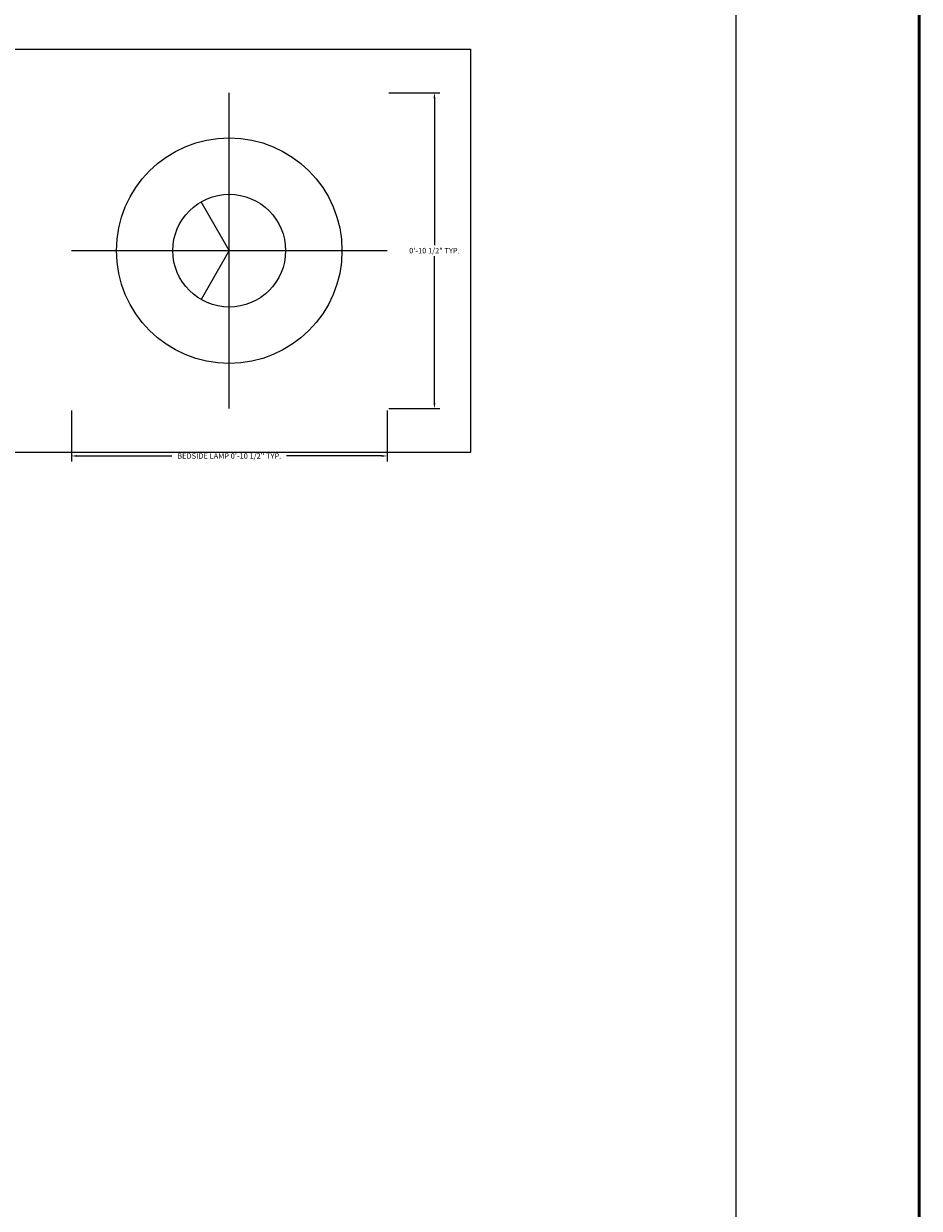
# Model space of a CAD drawing. Units: inches. Extents: x 0 to 281, y -535 to 46.
# Tile 20 of 22: x 127 to 156, y -36 to 3. Entities that reach past the tile are written whole.
import ezdxf

# ---------------------------------------------------------------- set-up
doc = ezdxf.new("R2010")
doc.units = ezdxf.units.IN
doc.header["$MEASUREMENT"] = 0
for name, color, linetype, lineweight in [('A-ANNO-DIMS', 2, 'Continuous', 18), ('A-FURN', 8, 'Continuous', 18), ('A-WALL', 7, 'Continuous', 50)]:
    doc.layers.add(name, color=color, linetype=linetype, lineweight=lineweight)
doc.styles.get("Standard").update_dxf_attribs({"font": 'arial.ttf'})
doc.dimstyles.get("Standard").update_dxf_attribs({"dimtxt": 0.18, "dimasz": 0.18, "dimexe": 0.18, "dimexo": 0.0625, "dimgap": 0.09, "dimtad": 0, "dimtih": 1, "dimtoh": 1, "dimdec": 0, "dimzin": 0, "dimdsep": 46, "dimlunit": 3, "dimtxsty": 'Standard', "dimcen": 0.09, "dimadec": 0, "dimazin": 0, "dimtfac": 1, "dimtdec": 0, "dimtofl": 0, "dimtmove": 0, "dimatfit": 3, "dimfxl": 1, "dimtolj": 1, "dimtzin": 0, "dimarcsym": 0})

# ---------------------------------------------------------------- blocks, each defined once
blk = doc.blocks.new('BEDSIDE-LAMP')
for p, q in [((5.174, 0), (5.174, 10.348)), ((0, 5.174), (10.348, 5.174))]:
    blk.add_line(p, q)
for points in [[(5.174, 5.174), (4.25, 6.774)], [(5.174, 5.174), (4.25, 3.574)]]:
    blk.add_lwpolyline(points)
for radius in [3.696, 1.848]:
    blk.add_circle((5.174, 5.174), radius)
blk = doc.blocks.new('*D36')
at = {"layer": 'A-ANNO-DIMS', "color": 0, "lineweight": -2, "transparency": 16777216}
for p, q in [((128.666, -10.092), (128.666, -11.761)), ((139.014, -10.092), (139.014, -11.761)), ((128.846, -11.581), (131.961, -11.581)), ((138.834, -11.581), (135.718, -11.581))]:
    blk.add_line(p, q, dxfattribs=at)
at = {"layer": 'A-ANNO-DIMS', "color": 0, "transparency": 16777216}
for points in [[(128.846, -11.551), (128.846, -11.611), (128.666, -11.581)], [(138.834, -11.551), (138.834, -11.611), (139.014, -11.581)]]:
    blk.add_solid(points, dxfattribs=at)
at = {"layer": 'Defpoints', "color": 0, "transparency": 16777216}
for p in [(128.666, -10.029), (139.014, -10.029), (139.014, -11.581)]:
    blk.add_point(p, dxfattribs=at)
at = {"layer": 'A-ANNO-DIMS', "color": 0, "transparency": 16777216, "insert": (133.84, -11.581), "char_height": 0.18, "attachment_point": 5}
blk.add_mtext('\\A1;BEDSIDE LAMP 0\'-10 1/2" TYP.', dxfattribs=at)
blk = doc.blocks.new('*D37')
at = {"layer": 'A-ANNO-DIMS', "color": 0, "lineweight": -2, "transparency": 16777216}
for p, q in [((139.076, 0.319), (140.746, 0.319)), ((140.566, 0.139), (140.566, -4.672)), ((140.566, -9.849), (140.566, -5.038)), ((139.076, -10.029), (140.746, -10.029))]:
    blk.add_line(p, q, dxfattribs=at)
at = {"layer": 'A-ANNO-DIMS', "color": 0, "transparency": 16777216}
for points in [[(140.536, 0.139), (140.596, 0.139), (140.566, 0.319)], [(140.536, -9.849), (140.596, -9.849), (140.566, -10.029)]]:
    blk.add_solid(points, dxfattribs=at)
at = {"layer": 'Defpoints', "color": 0, "transparency": 16777216}
for p in [(139.014, 0.319), (140.566, 0.319), (139.014, -10.029)]:
    blk.add_point(p, dxfattribs=at)
at = {"layer": 'A-ANNO-DIMS', "color": 0, "transparency": 16777216, "insert": (140.566, -4.855), "char_height": 0.18, "attachment_point": 5}
blk.add_mtext('\\A1;0\'-10 1/2" TYP.', dxfattribs=at)
blk = doc.blocks.new('*D45')
at = {"layer": 'A-ANNO-DIMS', "color": 0, "lineweight": -2, "transparency": 16777216}
for p, q in [((114.459, -263.348), (114.459, 46.219)), ((150.459, -263.348), (150.459, 46.219)), ((114.639, 46.039), (132.13, 46.039)), ((150.279, 46.039), (132.788, 46.039))]:
    blk.add_line(p, q, dxfattribs=at)
at = {"layer": 'A-ANNO-DIMS', "color": 0, "transparency": 16777216}
for points in [[(114.639, 46.069), (114.639, 46.009), (114.459, 46.039)], [(150.279, 46.069), (150.279, 46.009), (150.459, 46.039)]]:
    blk.add_solid(points, dxfattribs=at)
at = {"layer": 'Defpoints', "color": 0, "transparency": 16777216}
for p in [(150.459, 46.039), (114.459, -263.411), (150.459, -263.411)]:
    blk.add_point(p, dxfattribs=at)
at = {"layer": 'A-ANNO-DIMS', "color": 0, "transparency": 16777216, "insert": (132.459, 46.039), "char_height": 0.18, "attachment_point": 5}
blk.add_mtext('\\A1;3\'-0"', dxfattribs=at)
blk = doc.blocks.new('*D47')
at = {"layer": 'A-ANNO-DIMS', "color": 0, "lineweight": -2, "transparency": 16777216}
for p, q in [((114.459, -392.348), (114.459, 46.219)), ((150.459, -392.348), (150.459, 46.219)), ((114.639, 46.039), (132.13, 46.039)), ((150.279, 46.039), (132.788, 46.039))]:
    blk.add_line(p, q, dxfattribs=at)
at = {"layer": 'A-ANNO-DIMS', "color": 0, "transparency": 16777216}
for points in [[(114.639, 46.069), (114.639, 46.009), (114.459, 46.039)], [(150.279, 46.069), (150.279, 46.009), (150.459, 46.039)]]:
    blk.add_solid(points, dxfattribs=at)
at = {"layer": 'Defpoints', "color": 0, "transparency": 16777216}
for p in [(150.459, 46.039), (114.459, -392.411), (150.459, -392.411)]:
    blk.add_point(p, dxfattribs=at)
at = {"layer": 'A-ANNO-DIMS', "color": 0, "transparency": 16777216, "insert": (132.459, 46.039), "char_height": 0.18, "attachment_point": 5}
blk.add_mtext('\\A1;3\'-0"', dxfattribs=at)

msp = doc.modelspace()

# ---------------------------------------------------------------- linework, layer by layer
at = {"layer": 'A-FURN'}
msp.add_line((62.566, 1.744), (141.759, 1.744), dxfattribs=at)
msp.add_lwpolyline([(125.92, 1.744), (125.92, -11.454), (141.759, -11.454), (141.759, 1.744)], dxfattribs=at)
at = {"layer": 'A-WALL'}
msp.add_line((156.459, 18.589), (156.459, -131.411), dxfattribs=at)

# ---------------------------------------------------------------- block references
at = {"layer": 'A-FURN'}
msp.add_blockref('BEDSIDE-LAMP', (128.666, -10.029), dxfattribs=at)

# ---------------------------------------------------------------- dimensions: what is measured, and where the dimension line sits
at = {"layer": 'A-ANNO-DIMS'}
for p1, p2, picture in [((114.459, -263.411), (150.459, -263.411), '*D45'), ((114.459, -392.411), (150.459, -392.411), '*D47')]:
    dim = msp.add_linear_dim(base=(150.459, 46.039), p1=p1, p2=p2, dimstyle='Standard', override={"dimdec": 1, "dimlfac": 1, "dimrnd": 0, "dimzin": 1, "dimdsep": 46, "dimlunit": 4, "dimfrac": 2}, dxfattribs=at)
    dim.commit()
    dim.dimension.update_dxf_attribs({"geometry": picture, "text_midpoint": (132.459, 46.039)})
dim = msp.add_linear_dim(base=(140.566, 0.319), p1=(139.014, -10.029), p2=(139.014, 0.319), angle=90, text='<> TYP.', dimstyle='Standard', override={"dimdec": 1, "dimlfac": 1, "dimrnd": 0, "dimzin": 1, "dimdsep": 46, "dimlunit": 4, "dimfrac": 2}, dxfattribs=at)
dim.commit()
dim.dimension.update_dxf_attribs({"geometry": '*D37', "text_midpoint": (140.566, -4.855)})
dim = msp.add_linear_dim(base=(139.014, -11.581), p1=(128.666, -10.029), p2=(139.014, -10.029), text='BEDSIDE LAMP <> TYP.', dimstyle='Standard', override={"dimdec": 1, "dimlfac": 1, "dimrnd": 0, "dimzin": 1, "dimdsep": 46, "dimlunit": 4, "dimfrac": 2}, dxfattribs=at)
dim.commit()
dim.dimension.update_dxf_attribs({"geometry": '*D36', "text_midpoint": (133.84, -11.581)})

doc.saveas('drawing.dxf')
